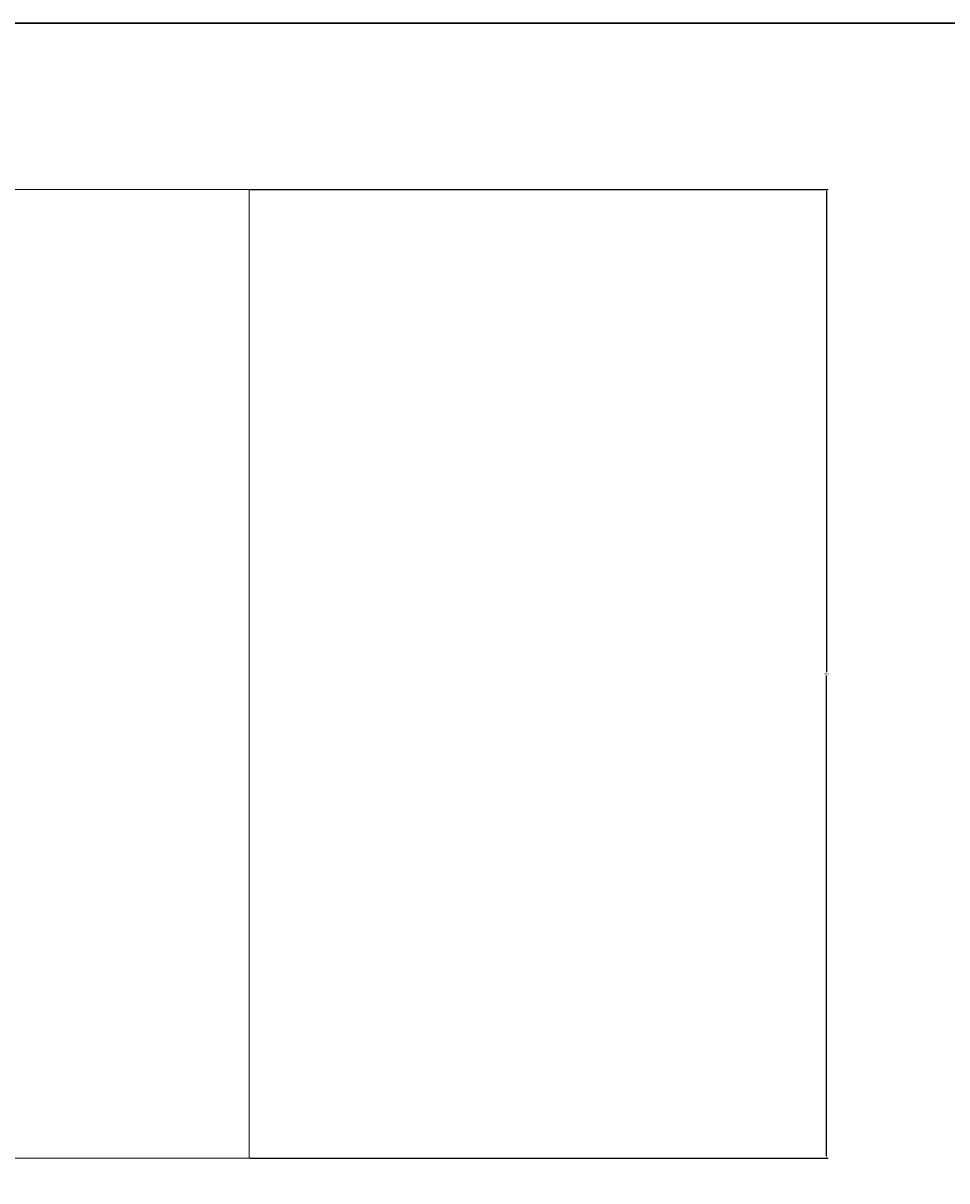
# Model space of a CAD drawing. Units: inches. Extents: x -46 to 1145, y -527 to 760.
# Tile 14 of 57: x 479 to 573, y -157 to -39. Entities that reach past the tile are written whole.
import ezdxf

# ---------------------------------------------------------------- set-up
doc = ezdxf.new("R2010")
doc.units = ezdxf.units.IN
doc.header["$MEASUREMENT"] = 0
for name, color, linetype, lineweight in [('A-ANNO-DIMS', 2, 'Continuous', 18), ('C-PKNG', 8, 'Continuous', 18), ('C-SITE', 7, 'Continuous', 30)]:
    doc.layers.add(name, color=color, linetype=linetype, lineweight=lineweight)
doc.styles.get("Standard").update_dxf_attribs({"font": 'arial.ttf'})
doc.dimstyles.get("Standard").update_dxf_attribs({"dimtxt": 0.18, "dimasz": 0.18, "dimexe": 0.18, "dimexo": 0.0625, "dimgap": 0.09, "dimtad": 0, "dimtih": 1, "dimtoh": 1, "dimdec": 0, "dimzin": 0, "dimdsep": 46, "dimlunit": 3, "dimtxsty": 'Standard', "dimcen": 0.09, "dimadec": 0, "dimazin": 0, "dimtfac": 1, "dimtdec": 0, "dimtofl": 0, "dimtmove": 0, "dimatfit": 3, "dimfxl": 1, "dimtolj": 1, "dimtzin": 0, "dimarcsym": 0})

# ---------------------------------------------------------------- blocks, each defined once
blk = doc.blocks.new('*D692')
at = {"layer": 'A-ANNO-DIMS', "color": 0, "lineweight": -2, "transparency": 16777216}
for p, q in [((501.79, -56.37), (560.51, -56.37)), ((560.33, -56.55), (560.33, -105.34)), ((560.33, -154.49), (560.33, -105.7)), ((501.79, -154.67), (560.51, -154.67))]:
    blk.add_line(p, q, dxfattribs=at)
at = {"layer": 'A-ANNO-DIMS', "color": 0, "transparency": 16777216}
for points in [[(560.3, -56.55), (560.36, -56.55), (560.33, -56.37)], [(560.3, -154.49), (560.36, -154.49), (560.33, -154.67)]]:
    blk.add_solid(points, dxfattribs=at)
at = {"layer": 'Defpoints', "color": 0, "transparency": 16777216}
for p in [(501.73, -56.37), (501.73, -154.67), (560.33, -154.67)]:
    blk.add_point(p, dxfattribs=at)
at = {"layer": 'A-ANNO-DIMS', "color": 0, "transparency": 16777216, "insert": (560.33, -105.52), "char_height": 0.18, "attachment_point": 5}
blk.add_mtext('\\A1;98.3', dxfattribs=at)
blk = doc.blocks.new('*D702')
at = {"layer": 'A-ANNO-DIMS', "color": 0, "lineweight": -2, "transparency": 16777216}
for p, q in [((189.63, -39.48), (1145.34, -39.48)), ((1145.16, -39.66), (1145.16, -249.3)), ((1145.16, -459.3), (1145.16, -249.66)), ((183.63, -459.48), (1145.34, -459.48))]:
    blk.add_line(p, q, dxfattribs=at)
at = {"layer": 'A-ANNO-DIMS', "color": 0, "transparency": 16777216}
for points in [[(1145.13, -39.66), (1145.19, -39.66), (1145.16, -39.48)], [(1145.13, -459.3), (1145.19, -459.3), (1145.16, -459.48)]]:
    blk.add_solid(points, dxfattribs=at)
at = {"layer": 'Defpoints', "color": 0, "transparency": 16777216}
for p in [(189.56, -39.48), (1145.16, -39.48), (183.56, -459.48)]:
    blk.add_point(p, dxfattribs=at)
at = {"layer": 'A-ANNO-DIMS', "color": 0, "transparency": 16777216, "insert": (1145.16, -249.48), "char_height": 0.18, "attachment_point": 5}
blk.add_mtext('\\A1;420', dxfattribs=at)

msp = doc.modelspace()

# ---------------------------------------------------------------- linework, layer by layer
at = {"layer": 'C-PKNG'}
msp.add_lwpolyline([(501.7297, -154.6684), (273.5156, -154.6684), (273.5156, -56.3706), (501.7297, -56.3706)], close=True, dxfattribs=at)
at = {"layer": 'C-SITE'}
msp.add_line((590.0637, -39.4824), (189.5637, -39.4824), dxfattribs=at)

# ---------------------------------------------------------------- dimensions: what is measured, and where the dimension line sits
at = {"layer": 'A-ANNO-DIMS'}
for base, p1, p2, angle, override, picture, middle in [((1145.1637, -39.4824), (183.5637, -459.4824), (189.5637, -39.4824), 90, {"dimdec": 0, "dimlfac": 1, "dimrnd": 0, "dimzin": 0, "dimdsep": 46, "dimlunit": 2}, '*D702', (1145.1637, -249.4824)), ((560.3297, -154.6684), (501.7297, -56.3706), (501.7297, -154.6684), 270, {"dimdec": 1, "dimlfac": 1, "dimrnd": 0, "dimzin": 0, "dimdsep": 46, "dimlunit": 2}, '*D692', (560.3297, -105.5195))]:
    dim = msp.add_linear_dim(base=base, p1=p1, p2=p2, angle=angle, dimstyle='Standard', override=override, dxfattribs=at)
    dim.commit()
    dim.dimension.update_dxf_attribs({"geometry": picture, "text_midpoint": middle})

doc.saveas('drawing.dxf')
